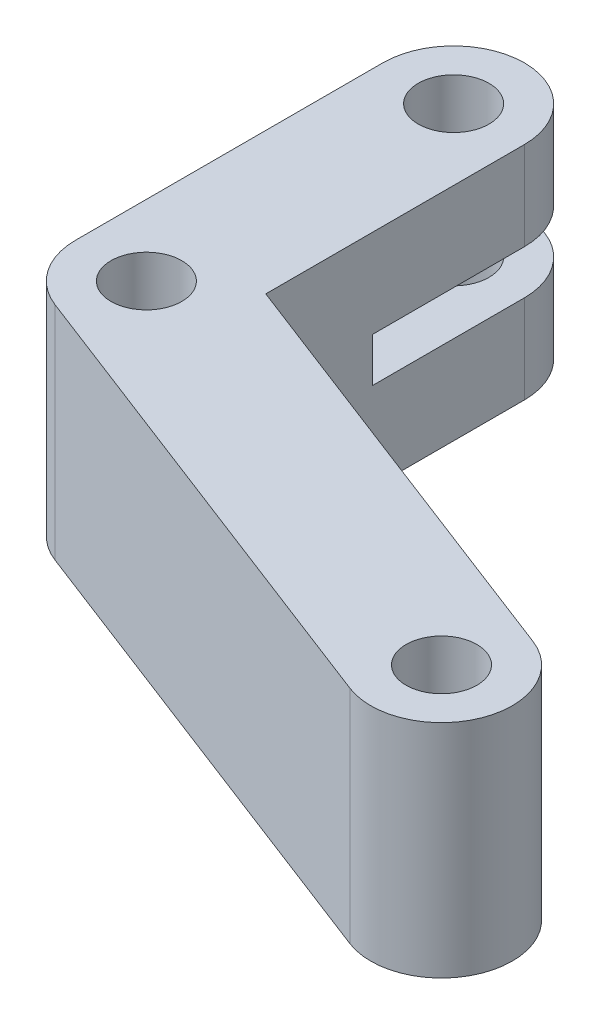
from build123d import *

# Parameters (mm, degrees)
L_BRACKET_BODY_DEPTH   = 25
PIVOT_HOLES_SKETCH_R   = 4
PIVOT_HOLES_3X_8_DEPTH = 25
CLEVIS_SLOT_SKETCH_W   = 25.15
CLEVIS_SLOT_SKETCH_H   = 5
CLEVIS_SLOT_5MM_DEPTH  = 12.5


with BuildPart() as part:
    # Bracket Profile Sketch → L Bracket Body (new body)
    with BuildSketch(Plane(origin=(0, 0, 0), x_dir=(1, 0, 0), z_dir=(0, 1, 0))):
        with BuildLine():
            Line((8, 34.72), (8, 5.491702761))
            Line((8, 5.491702761), (57.11524489, -13.424548452))
            ThreePointArc((57.11524489, -13.424548452), (61.705451548, -23.76524489), (51.36475511, -28.355451548))
            Line((51.36475511, -28.355451548), (-2.87524489, -7.465451548))
            ThreePointArc((-2.87524489, -7.465451548), (-6.595527239, -4.527584393), (-8, 0))
            Line((-8, 0), (-8, 34.72))
            ThreePointArc((-8, 34.72), (0, 42.72), (8, 34.72))
        make_face()
    extrude(amount=L_BRACKET_BODY_DEPTH)

    # Pivot Holes Sketch → Pivot Holes 3xØ8 (cut)
    with BuildSketch(Plane(origin=(0, 25, 0), x_dir=(1, 0, 0), z_dir=(0, 1, 0))):
        with Locations(Location((0, 34.72, 0), (0, 0, 270))):
            Circle(PIVOT_HOLES_SKETCH_R)
        with Locations(Location((54.24, -20.89, 0), (0, 0, 270))):
            Circle(PIVOT_HOLES_SKETCH_R)
        with Locations(Location((0, 0, 0), (0, 0, 270))):
            Circle(PIVOT_HOLES_SKETCH_R)
    extrude(amount=-PIVOT_HOLES_3X_8_DEPTH, mode=Mode.SUBTRACT)

    # Clevis Slot Sketch → Clevis Slot 5mm (cut, symmetric)
    with BuildSketch(Plane(origin=(0, 0, 0), x_dir=(0, 0, -1), z_dir=(1, 0, 0))):
        with Locations((30.145, 12.5)):
            Rectangle(CLEVIS_SLOT_SKETCH_W, CLEVIS_SLOT_SKETCH_H)
    extrude(amount=CLEVIS_SLOT_5MM_DEPTH, both=True, mode=Mode.SUBTRACT)


solid = part.part
